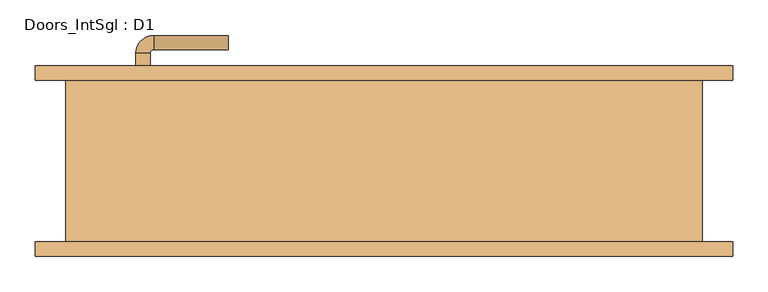
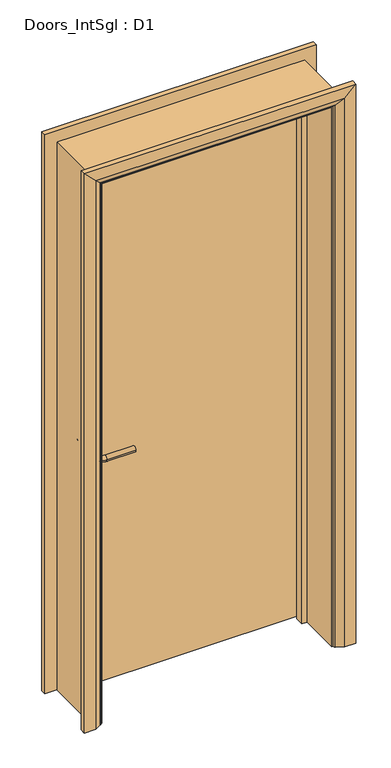
"""IFC4 building model written with IfcOpenShell, lengths in millimetres: door geometry, Doors_IntSgl : D1."""

from ifc_helpers import new_model, si_unit, point, frame, frame_2d, origin, place, context, project, spatial, polyline, circle_curve, ellipse_curve, trimmed, segment, composite_curve, outline, extrude, faceted_brep, source, transform, mapped, element, save
from ifc_brep_helpers import plane_surface, cylinder_surface, revolved_surface, advanced_brep


def doors_intsgl_d1_91024936(model_context):
    return source(origin(), model_context, "Body", "SolidModel", [
        advanced_brep(
        [(-350.2, 68.3, 900.0), (-330.2, 68.3, 900.0), (-330.2, 38.3, 900.0), (-350.2, 38.3, 900.0), (-325.2, 33.3, 900.0), (-325.2, 13.3, 900.0), (-220.2, 13.3, 900.0), (-220.2, 33.3, 900.0)],
        [
            (0, 1, circle_curve(frame((-340.2, 68.3, 900.0), z_axis=(0.0, 1.0, 0.0), x_axis=(1.0, 0.0, 0.0)), 10.0)),
            (1, 0, circle_curve(frame((-340.2, 68.3, 900.0), z_axis=(0.0, 1.0, 0.0), x_axis=(1.0, 0.0, 0.0)), 10.0)),
            (1, 2),
            (2, 3, circle_curve(frame((-340.2, 38.3, 900.0), z_axis=(0.0, 1.0, 0.0), x_axis=(1.0, 0.0, 0.0)), 10.0)),
            (3, 0),
            (3, 2, circle_curve(frame((-340.2, 38.3, 900.0), z_axis=(0.0, 1.0, 0.0), x_axis=(1.0, 0.0, 0.0)), 10.0)),
            (4, 5, circle_curve(frame((-325.2, 23.3, 900.0), z_axis=(-1.0, 0.0, 0.0), x_axis=(0.0, 1.0, 0.0)), 10.0)),
            (5, 3, circle_curve(frame((-325.2, 38.3, 900.0), z_axis=(0.0, 0.0, -1.0), x_axis=(-1.0, 0.0, 0.0)), 25.0)),
            (2, 4, circle_curve(frame((-325.2, 38.3, 900.0), z_axis=(0.0, 0.0, 1.0), x_axis=(-1.0, 0.0, 0.0)), 5.0)),
            (5, 4, circle_curve(frame((-325.2, 23.3, 900.0), z_axis=(-1.0, 0.0, 0.0), x_axis=(0.0, 1.0, 0.0)), 10.0)),
            (6, 7, circle_curve(frame((-220.2, 23.3, 900.0), z_axis=(1.0, 0.0, 0.0), x_axis=(0.0, 1.0, 0.0)), 10.0)),
            (7, 6, circle_curve(frame((-220.2, 23.3, 900.0), z_axis=(1.0, 0.0, 0.0), x_axis=(0.0, 1.0, 0.0)), 10.0)),
            (4, 7),
            (6, 5),
        ],
        [
            plane_surface(frame((-340.2, 68.3, 900.0), z_axis=(0.0, 1.0, 0.0), x_axis=(0.0, 0.0, 1.0))),
            cylinder_surface(frame((-340.2, 68.3, 900.0), z_axis=(0.0, 1.0, 0.0), x_axis=(1.0, 0.0, 0.0)), 10.0),
            revolved_surface(trimmed(ellipse_curve(frame((-340.2, 38.3, 900.0), z_axis=(0.0, -1.0, 0.0), x_axis=(1.0, 0.0, 0.0)), 10.0, 10.0), [point((-350.2, 38.3, 900.0))], [point((-330.2, 38.3, 900.0))], True, "CARTESIAN"), (-325.2, 38.3, 900.0), (0.0, 0.0, -1.0)),
            revolved_surface(trimmed(ellipse_curve(frame((-340.2, 38.3, 900.0), z_axis=(0.0, -1.0, 0.0), x_axis=(1.0, 0.0, 0.0)), 10.0, 10.0), [point((-330.2, 38.3, 900.0))], [point((-350.2, 38.3, 900.0))], True, "CARTESIAN"), (-325.2, 38.3, 900.0), (0.0, 0.0, -1.0)),
            plane_surface(frame((-220.2, 23.3, 900.0), z_axis=(1.0, 0.0, 0.0), x_axis=(0.0, 0.0, 1.0))),
            cylinder_surface(frame((-325.2, 23.3, 900.0), z_axis=(-1.0, 0.0, 0.0), x_axis=(0.0, 1.0, 0.0)), 10.0),
        ],
        [
            (0, [[1, 2]]),
            (1, [[3, 4, 5, -2]]),
            (1, [[-5, 6, -3, -1]]),
            (2, [[7, 8, -4, 9]]),
            (3, [[10, -9, -6, -8]]),
            (4, [[11, 12]]),
            (5, [[13, -11, 14, -7]]),
            (5, [[-14, -12, -13, -10]]),
        ],
    ),
        extrude(outline(composite_curve([segment(trimmed(circle_curve(frame_2d((900.0, -342.7)), 30.0), [point((900.0, -372.7))], [point((900.0, -312.7))], False, "CARTESIAN"), True, "CONTINUOUS"), segment(trimmed(circle_curve(frame_2d((900.0, -342.7)), 30.0), [point((900.0, -312.7))], [point((900.0, -372.7))], False, "CARTESIAN"), True, "CONTINUOUS")], self_intersect=False)), frame((0.0, 68.3, 0.0), z_axis=(0.0, 1.0, 0.0), x_axis=(0.0, 0.0, 1.0)), (0.0, 0.0, 1.0), 8.0),
        advanced_brep(
        [(-350.2, 122.3, 900.0), (-330.2, 122.3, 900.0), (-350.2, 152.3, 900.0), (-330.2, 152.3, 900.0), (-325.2, 157.3, 900.0), (-325.2, 177.3, 900.0), (-220.2, 177.3, 900.0), (-220.2, 157.3, 900.0)],
        [
            (0, 1, circle_curve(frame((-340.2, 122.3, 900.0), z_axis=(0.0, -1.0, 0.0), x_axis=(1.0, 0.0, 0.0)), 10.0)),
            (1, 0, circle_curve(frame((-340.2, 122.3, 900.0), z_axis=(0.0, -1.0, 0.0), x_axis=(1.0, 0.0, 0.0)), 10.0)),
            (0, 2),
            (2, 3, circle_curve(frame((-340.2, 152.3, 900.0), z_axis=(0.0, -1.0, 0.0), x_axis=(1.0, 0.0, 0.0)), 10.0)),
            (3, 1),
            (3, 2, circle_curve(frame((-340.2, 152.3, 900.0), z_axis=(0.0, -1.0, 0.0), x_axis=(1.0, 0.0, 0.0)), 10.0)),
            (4, 3, circle_curve(frame((-325.2, 152.3, 900.0), z_axis=(0.0, 0.0, 1.0), x_axis=(-1.0, 0.0, 0.0)), 5.0)),
            (2, 5, circle_curve(frame((-325.2, 152.3, 900.0), z_axis=(0.0, 0.0, -1.0), x_axis=(-1.0, 0.0, 0.0)), 25.0)),
            (5, 4, circle_curve(frame((-325.2, 167.3, 900.0), z_axis=(-1.0, 0.0, 0.0), x_axis=(0.0, -1.0, 0.0)), 10.0)),
            (4, 5, circle_curve(frame((-325.2, 167.3, 900.0), z_axis=(-1.0, 0.0, 0.0), x_axis=(0.0, -1.0, 0.0)), 10.0)),
            (6, 7, circle_curve(frame((-220.2, 167.3, 900.0), z_axis=(1.0, 0.0, 0.0), x_axis=(0.0, -1.0, 0.0)), 10.0)),
            (7, 6, circle_curve(frame((-220.2, 167.3, 900.0), z_axis=(1.0, 0.0, 0.0), x_axis=(0.0, -1.0, 0.0)), 10.0)),
            (5, 6),
            (7, 4),
        ],
        [
            plane_surface(frame((-340.2, 122.3, 900.0), z_axis=(0.0, -1.0, 0.0), x_axis=(0.0, 0.0, 1.0))),
            cylinder_surface(frame((-340.2, 122.3, 900.0), z_axis=(0.0, -1.0, 0.0), x_axis=(1.0, 0.0, 0.0)), 10.0),
            revolved_surface(trimmed(ellipse_curve(frame((-340.2, 152.3, 900.0), z_axis=(0.0, -1.0, 0.0), x_axis=(1.0, 0.0, 0.0)), 10.0, 10.0), [point((-350.2, 152.3, 900.0))], [point((-330.2, 152.3, 900.0))], True, "CARTESIAN"), (-325.2, 152.3, 900.0), (0.0, 0.0, -1.0)),
            revolved_surface(trimmed(ellipse_curve(frame((-340.2, 152.3, 900.0), z_axis=(0.0, -1.0, 0.0), x_axis=(1.0, 0.0, 0.0)), 10.0, 10.0), [point((-330.2, 152.3, 900.0))], [point((-350.2, 152.3, 900.0))], True, "CARTESIAN"), (-325.2, 152.3, 900.0), (0.0, 0.0, -1.0)),
            plane_surface(frame((-220.2, 167.3, 900.0), z_axis=(1.0, 0.0, 0.0), x_axis=(0.0, 0.0, 1.0))),
            cylinder_surface(frame((-325.2, 167.3, 900.0), z_axis=(-1.0, 0.0, 0.0), x_axis=(0.0, -1.0, 0.0)), 10.0),
        ],
        [
            (0, [[1, 2]]),
            (1, [[-1, 3, 4, 5]]),
            (1, [[-2, -5, 6, -3]]),
            (2, [[7, -4, 8, 9]]),
            (3, [[-8, -6, -7, 10]]),
            (4, [[11, 12]]),
            (5, [[-9, 13, -12, 14]]),
            (5, [[-10, -14, -11, -13]]),
        ],
    ),
        extrude(outline(composite_curve([segment(trimmed(circle_curve(frame_2d((900.0, -342.7)), 30.0), [point((900.0, -372.7))], [point((900.0, -312.7))], False, "CARTESIAN"), True, "CONTINUOUS"), segment(trimmed(circle_curve(frame_2d((900.0, -342.7)), 30.0), [point((900.0, -312.7))], [point((900.0, -372.7))], False, "CARTESIAN"), True, "CONTINUOUS")], self_intersect=False)), frame((0.0, 114.3, 0.0), z_axis=(0.0, 1.0, 0.0), x_axis=(0.0, 0.0, 1.0)), (0.0, 0.0, 1.0), 8.0),
        extrude(outline(polyline([(415.2, 76.3), (-415.2, 76.3), (-415.2, 114.3), (415.2, 114.3), (415.2, 76.3)])), frame((0.0, 0.0, 8.0), z_axis=(0.0, 0.0, 1.0), x_axis=(1.0, 0.0, 0.0)), (0.0, 0.0, 1.0), 2060.0),
        advanced_brep(
        [(492.2, 134.3, 0.0), (492.2, 114.3, 0.0), (422.2, 114.3, 0.0), (426.2, 120.3, 0.0), (452.2, 134.3, 0.0), (492.2, 134.3, 2145.0), (492.2, 114.3, 2145.0), (-492.2, 114.3, 2145.0), (-492.2, 114.3, 0.0), (-422.2, 114.3, 0.0), (-422.2, 114.3, 2075.0), (422.2, 114.3, 2075.0), (426.2, 120.3, 2079.0), (452.2, 134.3, 2105.0), (-452.2, 134.3, 2105.0), (-452.2, 134.3, 0.0), (-492.2, 134.3, 0.0), (-492.2, 134.3, 2145.0), (-426.2, 120.3, 0.0), (-426.2, 120.3, 2079.0)],
        [
            (0, 1),
            (1, 2),
            (2, 3, circle_curve(frame((430.2, 113.3, 0.0), z_axis=(0.0, 0.0, -1.0), x_axis=(1.0, 0.0, 0.0)), 8.0622577)),
            (3, 4),
            (4, 0),
            (0, 5),
            (5, 6),
            (6, 1),
            (6, 7),
            (7, 8),
            (8, 9),
            (9, 10),
            (10, 11),
            (11, 2),
            (11, 12, ellipse_curve(frame((430.2, 113.3, 2083.0), z_axis=(0.7071067811865475, 0.0, -0.7071067811865475), x_axis=(-0.7071067811865474, 0.0, -0.7071067811865476)), 11.4017543, 8.0622577)),
            (12, 3),
            (12, 13),
            (13, 4),
            (13, 14),
            (14, 15),
            (15, 16),
            (16, 17),
            (17, 5),
            (7, 17),
            (16, 8),
            (15, 18),
            (18, 9, circle_curve(frame((-430.2, 113.3, 0.0), z_axis=(0.0, 0.0, -1.0), x_axis=(-1.0, 0.0, 0.0)), 8.0622577)),
            (19, 10, ellipse_curve(frame((-430.2, 113.3, 2083.0), z_axis=(-0.7071067811865475, 0.0, -0.7071067811865475), x_axis=(-0.7071067811865474, 0.0, 0.7071067811865476)), 11.4017543, 8.0622577)),
            (18, 19),
            (14, 19),
            (19, 12),
        ],
        [
            plane_surface(frame((422.2, 114.3, 0.0), z_axis=(0.0, 0.0, -1.0), x_axis=(0.0, -1.0, 0.0))),
            plane_surface(frame((492.2, 134.3, 0.0), z_axis=(1.0, 0.0, 0.0), x_axis=(0.0, 0.0, 1.0))),
            plane_surface(frame((492.2, 114.3, 0.0), z_axis=(0.0, -1.0, 0.0), x_axis=(0.0, 0.0, 1.0))),
            cylinder_surface(frame((430.2, 113.3, 0.0), z_axis=(0.0, 0.0, -1.0), x_axis=(1.0, 0.0, 0.0)), 8.0622577),
            plane_surface(frame((426.2, 120.3, 0.0), z_axis=(-0.4740998230350126, 0.880471099922178, 0.0), x_axis=(0.0, 0.0, 1.0))),
            plane_surface(frame((452.2, 134.3, 0.0), z_axis=(0.0, 1.0, 0.0), x_axis=(0.0, 0.0, 1.0))),
            plane_surface(frame((-492.2, 134.3, 2145.0), z_axis=(-1.0, 0.0, 0.0), x_axis=(0.0, 0.0, -1.0))),
            plane_surface(frame((-422.2, 114.3, 0.0), z_axis=(0.0, 0.0, -1.0), x_axis=(0.0, -1.0, 0.0))),
            cylinder_surface(frame((-430.2, 113.3, 2075.0), z_axis=(0.0, 0.0, 1.0), x_axis=(-1.0, 0.0, 0.0)), 8.0622577),
            plane_surface(frame((-426.2, 120.3, 2079.0), z_axis=(0.47409982303501824, 0.8804710999221749, 0.0), x_axis=(0.0, 0.0, -1.0))),
            plane_surface(frame((492.2, 134.3, 2145.0), z_axis=(0.0, 0.0, 1.0), x_axis=(-1.0, 0.0, 0.0))),
            cylinder_surface(frame((422.2, 113.3, 2083.0), z_axis=(1.0, 0.0, 0.0), x_axis=(0.0, 0.0, 1.0)), 8.0622577),
            plane_surface(frame((426.2, 120.3, 2079.0), z_axis=(0.0, 0.8804710999221764, -0.4740998230350154), x_axis=(-1.0, 0.0, 0.0))),
        ],
        [
            (0, [[1, 2, 3, 4, 5]]),
            (1, [[-1, 6, 7, 8]]),
            (2, [[-2, -8, 9, 10, 11, 12, 13, 14]]),
            (3, [[-3, -14, 15, 16]]),
            (4, [[-4, -16, 17, 18]]),
            (5, [[-5, -18, 19, 20, 21, 22, 23, -6]]),
            (6, [[24, -22, 25, -10]]),
            (7, [[-21, 26, 27, -11, -25]]),
            (8, [[28, -12, -27, 29]]),
            (9, [[30, -29, -26, -20]]),
            (10, [[-7, -23, -24, -9]]),
            (11, [[-15, -13, -28, 31]]),
            (12, [[-17, -31, -30, -19]]),
        ],
    ),
        extrude(outline(polyline([(0.0, -417.2), (0.0, -398.2), (2051.0, -398.2), (2051.0, 398.2), (0.0, 398.2), (0.0, 417.2), (2070.0, 417.2), (2070.0, -417.2), (0.0, -417.2)])), frame((0.0, 42.3, 0.0), z_axis=(0.0, 1.0, 0.0), x_axis=(0.0, 0.0, 1.0)), (0.0, 0.0, 1.0), 32.0),
        advanced_brep(
        [(-492.2, -134.3, 0.0), (-492.2, -114.3, 0.0), (-422.2, -114.3, 0.0), (-426.2, -120.3, 0.0), (-452.2, -134.3, 0.0), (-492.2, -134.3, 2145.0), (-492.2, -114.3, 2145.0), (-422.2, -114.3, 2075.0), (-426.2, -120.3, 2079.0), (-452.2, -134.3, 2105.0), (492.2, -134.3, 0.0), (452.2, -134.3, 0.0), (426.2, -120.3, 0.0), (422.2, -114.3, 0.0), (492.2, -114.3, 0.0), (492.2, -134.3, 2145.0), (452.2, -134.3, 2105.0), (426.2, -120.3, 2079.0), (422.2, -114.3, 2075.0), (492.2, -114.3, 2145.0)],
        [
            (0, 1),
            (1, 2),
            (2, 3, circle_curve(frame((-430.2, -113.3, 0.0), z_axis=(0.0, 0.0, -1.0), x_axis=(-1.0, 0.0, 0.0)), 8.0622577)),
            (3, 4),
            (4, 0),
            (0, 5),
            (5, 6),
            (6, 1),
            (6, 7),
            (7, 2),
            (7, 8, ellipse_curve(frame((-430.2, -113.3, 2083.0), z_axis=(-0.7071067811865475, 0.0, -0.7071067811865475), x_axis=(0.7071067811865474, 0.0, -0.7071067811865476)), 11.4017543, 8.0622577)),
            (8, 3),
            (8, 9),
            (9, 4),
            (9, 5),
            (10, 11),
            (11, 12),
            (12, 13, circle_curve(frame((430.2, -113.3, 0.0), z_axis=(0.0, 0.0, -1.0), x_axis=(1.0, 0.0, 0.0)), 8.0622577)),
            (13, 14),
            (14, 10),
            (15, 16),
            (16, 11),
            (10, 15),
            (16, 17),
            (17, 12),
            (17, 18, ellipse_curve(frame((430.2, -113.3, 2083.0), z_axis=(0.7071067811865475, 0.0, -0.7071067811865475), x_axis=(0.7071067811865474, 0.0, 0.7071067811865476)), 11.4017543, 8.0622577)),
            (18, 13),
            (18, 19),
            (19, 14),
            (19, 15),
            (5, 15),
            (19, 6),
            (18, 7),
            (17, 8),
            (16, 9),
        ],
        [
            plane_surface(frame((-422.2, -187.1010989, 0.0), z_axis=(0.0, 0.0, -1.0), x_axis=(1.0, 0.0, 0.0))),
            plane_surface(frame((-492.2, -134.3, 0.0), z_axis=(-1.0, 0.0, 0.0), x_axis=(0.0, 0.0, 1.0))),
            plane_surface(frame((-492.2, -114.3, 0.0), z_axis=(0.0, 1.0, 0.0), x_axis=(0.0, 0.0, 1.0))),
            cylinder_surface(frame((-430.2, -113.3, 0.0), z_axis=(0.0, 0.0, -1.0), x_axis=(-1.0, 0.0, 0.0)), 8.0622577),
            plane_surface(frame((-426.2, -120.3, 0.0), z_axis=(0.4740998230350183, -0.8804710999221749, 0.0), x_axis=(0.0, 0.0, 1.0))),
            plane_surface(frame((-452.2, -134.3, 0.0), z_axis=(0.0, -1.0, 0.0), x_axis=(0.0, 0.0, 1.0))),
            plane_surface(frame((422.2, -187.1010989, 0.0), z_axis=(0.0, 0.0, -1.0), x_axis=(-1.0, 0.0, 0.0))),
            plane_surface(frame((452.2, -134.3, 2105.0), z_axis=(0.0, -1.0, 0.0), x_axis=(0.0, 0.0, -1.0))),
            plane_surface(frame((426.2, -120.3, 2079.0), z_axis=(-0.4740998230350183, -0.8804710999221749, 0.0), x_axis=(0.0, 0.0, -1.0))),
            cylinder_surface(frame((430.2, -113.3, 2075.0), z_axis=(0.0, 0.0, 1.0), x_axis=(1.0, 0.0, 0.0)), 8.0622577),
            plane_surface(frame((492.2, -114.3, 2145.0), z_axis=(0.0, 1.0, 0.0), x_axis=(0.0, 0.0, -1.0))),
            plane_surface(frame((492.2, -134.3, 2145.0), z_axis=(1.0, 0.0, 0.0), x_axis=(0.0, 0.0, -1.0))),
            plane_surface(frame((-492.2, -134.3, 2145.0), z_axis=(0.0, 0.0, 1.0), x_axis=(1.0, 0.0, 0.0))),
            plane_surface(frame((-492.2, -114.3, 2145.0), z_axis=(0.0, 1.0, 0.0), x_axis=(1.0, 0.0, 0.0))),
            cylinder_surface(frame((-422.2, -113.3, 2083.0), z_axis=(-1.0, 0.0, 0.0), x_axis=(0.0, 0.0, 1.0)), 8.0622577),
            plane_surface(frame((-426.2, -120.3, 2079.0), z_axis=(0.0, -0.8804710999221749, -0.4740998230350183), x_axis=(1.0, 0.0, 0.0))),
            plane_surface(frame((-452.2, -134.3, 2105.0), z_axis=(0.0, -1.0, 0.0), x_axis=(1.0, 0.0, 0.0))),
        ],
        [
            (0, [[1, 2, 3, 4, 5]]),
            (1, [[-1, 6, 7, 8]]),
            (2, [[-2, -8, 9, 10]]),
            (3, [[-3, -10, 11, 12]]),
            (4, [[-4, -12, 13, 14]]),
            (5, [[-5, -14, 15, -6]]),
            (6, [[16, 17, 18, 19, 20]]),
            (7, [[21, 22, -16, 23]]),
            (8, [[24, 25, -17, -22]]),
            (9, [[26, 27, -18, -25]]),
            (10, [[28, 29, -19, -27]]),
            (11, [[30, -23, -20, -29]]),
            (12, [[-7, 31, -30, 32]]),
            (13, [[-9, -32, -28, 33]]),
            (14, [[-11, -33, -26, 34]]),
            (15, [[-13, -34, -24, 35]]),
            (16, [[-15, -35, -21, -31]]),
        ],
    ),
        faceted_brep([(-417.2, 114.3, 0.0), (-417.2, -114.3, 0.0), (-449.2, -114.3, 0.0), (-449.2, 114.3, 0.0), (-417.2, 114.3, 2070.0), (-417.2, -114.3, 2070.0), (-449.2, -114.3, 2102.0), (-449.2, 114.3, 2102.0), (417.2, 114.3, 0.0), (449.2, 114.3, 0.0), (449.2, -114.3, 0.0), (417.2, -114.3, 0.0), (417.2, 114.3, 2070.0), (449.2, 114.3, 2102.0), (449.2, -114.3, 2102.0), (417.2, -114.3, 2070.0)], [[[0, 1, 2, 3]], [[1, 0, 4, 5]], [[2, 1, 5, 6]], [[3, 2, 6, 7]], [[0, 3, 7, 4]], [[8, 9, 10, 11]], [[12, 13, 9, 8]], [[13, 14, 10, 9]], [[14, 15, 11, 10]], [[15, 12, 8, 11]], [[5, 4, 12, 15]], [[6, 5, 15, 14]], [[7, 6, 14, 13]], [[4, 7, 13, 12]]]),
    ])


if __name__ == "__main__":
    model = new_model("IFC4")
    model_context = context("Model", 3, world=origin())
    ifc_project = project(units=[si_unit("LENGTHUNIT", "METRE", prefix="MILLI")], contexts=[model_context])
    site = spatial("IfcSite", under=ifc_project)
    building = spatial("IfcBuilding", under=site)
    placement = place(None, origin())
    doors_intsgl_d1_shape = doors_intsgl_d1_91024936(model_context)
    element("IfcDoor", 1, ObjectType="Doors_IntSgl : D1", at=placement, inside=building, context=model_context, shape_type="MappedRepresentation", body=[
        mapped(doors_intsgl_d1_shape, transform((0.0, 0.0, 0.0), x_axis=(1.0, 0.0, 0.0), y_axis=(0.0, 1.0, 0.0), z_axis=(0.0, 0.0, 1.0))),
    ])
    save(model, "model.ifc")

# Revit data of these elements
# Type "Doors_IntSgl : D1"
#   Type Mark = "46"
#   Type Comments = "Internal Single"
#   Operation = "SingleSwingRight"
#   Manufacturer = "Revit"
#   Keynote = "L20"
#   Description = "Internal Single Door"
#   Analytic Construction = "Metal"
#   UnderCut = 0.026247 ft
#   Tolerance = 0.006562 ft
#   Thickness = 0.124672 ft
#   Thermal Resistance (R) = 0.270117 (m²·K)/W
#   Structural Tolerance = 0.026247 ft
#   StopDepth = 0.104987 ft
#   Stop Thickness = 0.062336 ft
#   Rough Width = 3.0 ft
#   Rough Height = 6.922572 ft
#   Height to Top Lock Rail = 3.28084 ft
#   Heat Transfer Coefficient (U) = 3.7021 W/(m²·K)
#   Handle Z Distance = 2.952756 ft
#   Handle X Distance = 0.246063 ft
#   Frame Thickness = 0.104987 ft
#   Door Panel Width = 2.724409 ft
#   Door Panel Thickness = 0.124672 ft
#   Door Panel Offset = 0.0 ft
#   Height = 6.922572 ft
#   Width = 3.0 ft
#   Door Panel Height = 6.75853 ft
#   Architrave Setback = 0.016404 ft
#   Vis - Ironmongery = yes
#   Material Ironmongery = Door - Handle
#   Material Frame = Door - Frame/Mullion (1)
#   Material Door = Door - Panel
#   Material Architrave = Door - Architrave
#   Visual Light Transmittance = 0
#   Solar Heat Gain Coefficient = 0
#   Function = (empty or 0)
#   Wall Closure = (empty or 0)
# Element 1 (IfcDoor, "Doors_IntSgl : D1")
#   Materials on its faces: "Door - Architrave", "Door - Handle", "Door - Frame/Mullion (1)", "Door - Panel"
# Materials
#   "Door - Handle": colour RGB 0 0 0, transparency 0, Keynote = "P21", Cost = 0
#   "Door - Frame/Mullion (1)": class "Wood", colour RGB 212 179 113, transparency 0, Keynote = "L20", Cost = 0
#   "Door - Panel": class "Wood", colour RGB 210 159 95, transparency 0, Keynote = "L20", Cost = 0
#   "Door - Architrave": class "Wood", colour RGB 154 90 5, transparency 0, Keynote = "P20", Cost = 0
